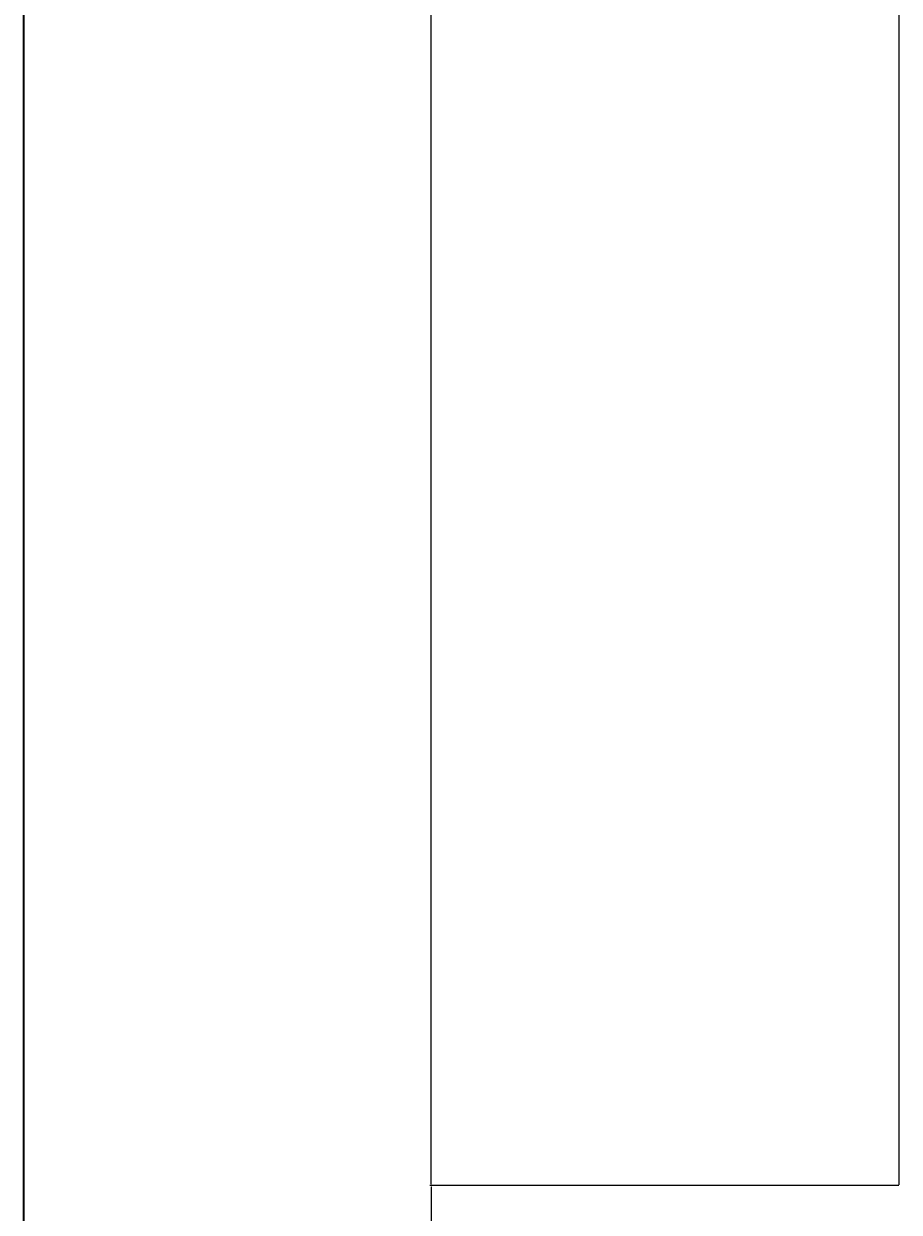
# Model space of a CAD drawing. Units: inches. Extents: x 1962 to 2771, y 1245 to 2660.
# Tile 37 of 114: x 1962 to 2072, y 2030 to 2180. Entities that reach past the tile are written whole.
import ezdxf

# ---------------------------------------------------------------- set-up
doc = ezdxf.new("R2010")
doc.units = ezdxf.units.IN
doc.layers.add('A-ANNO-DIMS', color=2, linetype='Continuous', lineweight=18)
doc.layers.add('A-ANNO-TTLB', color=7, linetype='Continuous', lineweight=35)
doc.styles.get("Standard").update_dxf_attribs({"font": 'arial.ttf'})
doc.dimstyles.get("Standard").update_dxf_attribs({"dimtxt": 0.18, "dimasz": 0.18, "dimexe": 0.18, "dimexo": 0.0625, "dimgap": 0.09, "dimtad": 0, "dimtih": 1, "dimtoh": 1, "dimdec": 4, "dimzin": 0, "dimdsep": 46, "dimtxsty": 'Standard', "dimcen": 0.09, "dimadec": 0, "dimazin": 0, "dimtfac": 1, "dimtdec": 4, "dimtofl": 0, "dimtmove": 0, "dimatfit": 3, "dimfxl": 1, "dimtolj": 1, "dimtzin": 0, "dimarcsym": 0})

# ---------------------------------------------------------------- blocks, each defined once
blk = doc.blocks.new('*D40')
at = {"layer": 'A-ANNO-DIMS', "color": 0, "lineweight": -2, "transparency": 16777216}
for p, q in [((2072.02, 2033.91), (2072.02, 2583.47)), ((2072.2, 2583.29), (2366.02, 2583.29)), ((2660.63, 2583.29), (2366.81, 2583.29)), ((2660.81, 2524.41), (2660.81, 2583.47))]:
    blk.add_line(p, q, dxfattribs=at)
at = {"layer": 'A-ANNO-DIMS', "color": 0, "transparency": 16777216}
for points in [[(2072.2, 2583.32), (2072.2, 2583.26), (2072.02, 2583.29)], [(2660.63, 2583.32), (2660.63, 2583.26), (2660.81, 2583.29)]]:
    blk.add_solid(points, dxfattribs=at)
at = {"layer": 'Defpoints', "color": 0, "transparency": 16777216}
for p in [(2660.81, 2583.29), (2660.81, 2524.34), (2072.02, 2033.84)]:
    blk.add_point(p, dxfattribs=at)
at = {"layer": 'A-ANNO-DIMS', "color": 0, "transparency": 16777216, "insert": (2366.41, 2583.29), "char_height": 0.18, "attachment_point": 5}
blk.add_mtext('\\A1;588.8', dxfattribs=at)
blk = doc.blocks.new('*D43')
at = {"layer": 'A-ANNO-DIMS', "color": 0, "lineweight": -2, "transparency": 16777216}
for p, q in [((2086.24, 2524.34), (2012.89, 2524.34)), ((2013.07, 2524.16), (2013.07, 2279.28)), ((2013.07, 2034.02), (2013.07, 2278.91)), ((2071.96, 2033.84), (2012.89, 2033.84))]:
    blk.add_line(p, q, dxfattribs=at)
at = {"layer": 'A-ANNO-DIMS', "color": 0, "transparency": 16777216}
for points in [[(2013.04, 2524.16), (2013.1, 2524.16), (2013.07, 2524.34)], [(2013.04, 2034.02), (2013.1, 2034.02), (2013.07, 2033.84)]]:
    blk.add_solid(points, dxfattribs=at)
at = {"layer": 'Defpoints', "color": 0, "transparency": 16777216}
for p in [(2086.31, 2524.34), (2013.07, 2033.84), (2072.02, 2033.84)]:
    blk.add_point(p, dxfattribs=at)
at = {"layer": 'A-ANNO-DIMS', "color": 0, "transparency": 16777216, "insert": (2013.07, 2279.09), "char_height": 0.18, "attachment_point": 5}
blk.add_mtext('\\A1;490.5', dxfattribs=at)
blk = doc.blocks.new('*D44')
at = {"layer": 'A-ANNO-DIMS', "color": 0, "lineweight": -2, "transparency": 16777216}
for p, q in [((2071.96, 2033.84), (2012.89, 2033.84)), ((2013.07, 2033.66), (2013.07, 1981.53)), ((2013.07, 1929.02), (2013.07, 1981.16)), ((2071.96, 1928.84), (2012.89, 1928.84))]:
    blk.add_line(p, q, dxfattribs=at)
at = {"layer": 'A-ANNO-DIMS', "color": 0, "transparency": 16777216}
for points in [[(2013.04, 2033.66), (2013.1, 2033.66), (2013.07, 2033.84)], [(2013.04, 1929.02), (2013.1, 1929.02), (2013.07, 1928.84)]]:
    blk.add_solid(points, dxfattribs=at)
at = {"layer": 'Defpoints', "color": 0, "transparency": 16777216}
for p in [(2072.02, 2033.84), (2013.07, 1928.84), (2072.02, 1928.84)]:
    blk.add_point(p, dxfattribs=at)
at = {"layer": 'A-ANNO-DIMS', "color": 0, "transparency": 16777216, "insert": (2013.07, 1981.34), "char_height": 0.18, "attachment_point": 5}
blk.add_mtext('\\A1;105', dxfattribs=at)

msp = doc.modelspace()

# ---------------------------------------------------------------- linework, layer by layer
at = {"layer": 'A-ANNO-TTLB'}
msp.add_lwpolyline([(1961.7365, 2660.2579), (2771.213, 2660.2579), (2771.213, 1244.5817), (1961.7365, 1244.5817)], close=True, dxfattribs=at)

# ---------------------------------------------------------------- dimensions: what is measured, and where the dimension line sits
at = {"layer": 'A-ANNO-DIMS'}
dim = msp.add_linear_dim(base=(2660.8074, 2583.2937), p1=(2072.0204, 2033.8437), p2=(2660.8074, 2524.3437), dimstyle='Standard', override={"dimdec": 1, "dimlfac": 1, "dimrnd": 0, "dimzin": 0, "dimdsep": 46, "dimlunit": 2}, dxfattribs=at)
dim.commit()
dim.dimension.update_dxf_attribs({"geometry": '*D40', "text_midpoint": (2366.4139, 2583.2937)})
for base, p1, p2, override, picture, middle in [((2013.0704, 2033.8437), (2086.3074, 2524.3437), (2072.0204, 2033.8437), {"dimdec": 1, "dimlfac": 1, "dimrnd": 0, "dimzin": 0, "dimdsep": 46, "dimlunit": 2}, '*D43', (2013.0704, 2279.0937)), ((2013.0704, 1928.8437), (2072.0204, 2033.8437), (2072.0204, 1928.8437), {"dimdec": 0, "dimlfac": 1, "dimrnd": 0, "dimzin": 0, "dimdsep": 46, "dimlunit": 2}, '*D44', (2013.0704, 1981.3437))]:
    dim = msp.add_linear_dim(base=base, p1=p1, p2=p2, angle=90, dimstyle='Standard', override=override, dxfattribs=at)
    dim.commit()
    dim.dimension.update_dxf_attribs({"geometry": picture, "text_midpoint": middle})

doc.saveas('drawing.dxf')
